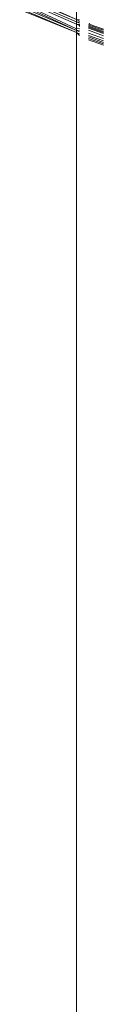
# Model space of a CAD drawing. Units: inches. Extents: x 64 to 1167, y 117 to 939.
# Tile 40 of 56: x 1129.775 to 1129.862, y 498.834 to 499.913. Entities that reach past the tile are written whole.
import ezdxf

# ---------------------------------------------------------------- set-up
doc = ezdxf.new("R2010")
doc.units = ezdxf.units.IN
doc.header["$MEASUREMENT"] = 0
doc.layers.add('A-FLOR-FIXT', color=8, linetype='Continuous', lineweight=18)

msp = doc.modelspace()

# ---------------------------------------------------------------- linework, layer by layer
at = {"layer": 'A-FLOR-FIXT'}
for p, q in [((1129.7801, 499.9332), (1129.8319, 499.9108)), ((1129.7811, 499.9352), (1129.8319, 499.9133)), ((1129.7816, 499.9363), (1129.8319, 499.9133)), ((1129.8319, 499.9362), (1129.8319, 499.9133)), ((1129.7749, 499.9222), (1129.8319, 499.8991)), ((1129.7755, 499.9235), (1129.8319, 499.8991)), ((1129.7764, 499.9253), (1129.8319, 499.9013)), ((1129.7771, 499.9268), (1129.8319, 499.9013)), ((1129.7779, 499.9284), (1129.8319, 499.9031)), ((1129.7792, 499.9312), (1129.8319, 499.9084)), ((1129.8319, 499.9133), (1129.8352, 499.9131)), ((1129.8319, 499.9133), (1129.8352, 499.9118)), ((1129.8319, 499.9108), (1129.8319, 499.9133)), ((1129.8319, 499.9108), (1129.8352, 499.9093)), ((1129.8319, 499.9108), (1129.8352, 499.9106)), ((1129.8319, 499.9084), (1129.8319, 499.9108)), ((1129.8319, 499.9084), (1129.8352, 499.907)), ((1129.8319, 499.9084), (1129.8352, 499.9081)), ((1129.8319, 499.9031), (1129.8319, 499.9084)), ((1129.8319, 499.9031), (1129.8352, 499.9036)), ((1129.8319, 499.9013), (1129.8319, 499.9031)), ((1129.8319, 499.9013), (1129.8352, 499.9016)), ((1129.8319, 499.9013), (1129.8352, 499.8999)), ((1129.8319, 499.8991), (1129.8319, 499.9013)), ((1129.8352, 499.9081), (1129.8352, 499.9058)), ((1129.8452, 499.9063), (1129.8616, 499.9004)), ((1129.8452, 499.9051), (1129.8616, 499.8992)), ((1129.8452, 499.9039), (1129.8616, 499.898)), ((1129.8452, 499.9016), (1129.8616, 499.8957)), ((1129.8453, 499.9074), (1129.8457, 499.9085)), ((1129.8453, 499.9074), (1129.8616, 499.9016)), ((1129.8457, 499.9085), (1129.8461, 499.9096)), ((1129.8457, 499.9085), (1129.8616, 499.9028)), ((1129.8319, 499.8991), (1129.8352, 499.8977)), ((1129.8319, 499.8991), (1129.8352, 499.8961)), ((1129.8319, 499.8991), (1129.8319, 495.6188)), ((1129.8452, 499.8985), (1129.8616, 499.8926)), ((1129.8452, 499.8958), (1129.8616, 499.8899)), ((1129.8452, 499.8943), (1129.8616, 499.8884)), ((1129.8452, 499.8926), (1129.8616, 499.8867)), ((1129.8452, 499.8913), (1129.8616, 499.8854))]:
    msp.add_line(p, q, dxfattribs=at)

doc.saveas('drawing.dxf')
